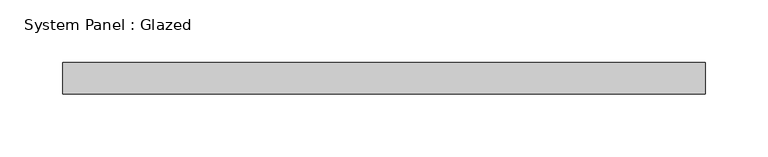
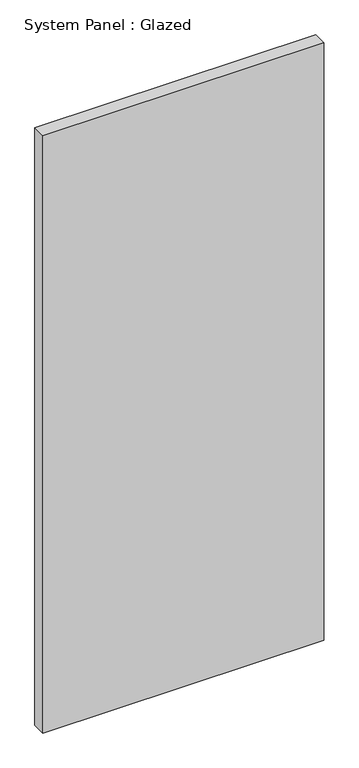
"""IFC4 building model written with IfcOpenShell, lengths in millimetres: plate geometry, System Panel : Glazed."""

from ifc_helpers import new_model, si_unit, origin, origin_with_axes, place, context, project, spatial, polyline, outline, extrude, source, transform, mapped, element, save


def system_panel_glazed_17912afe(model_context):
    return source(origin(), model_context, "Body", "SweptSolid", [
        extrude(outline(polyline([(257.175, 19.05), (-257.175, 19.05), (-257.175, 44.45), (257.175, 44.45), (257.175, 19.05)])), origin_with_axes(), (0.0, 0.0, 1.0), 1155.7),
    ])


if __name__ == "__main__":
    model = new_model("IFC4")
    model_context = context("Model", 3, world=origin())
    ifc_project = project(units=[si_unit("LENGTHUNIT", "METRE", prefix="MILLI")], contexts=[model_context])
    site = spatial("IfcSite", under=ifc_project)
    building = spatial("IfcBuilding", under=site)
    placement = place(None, origin())
    system_panel_glazed_shape = system_panel_glazed_17912afe(model_context)
    element("IfcPlate", 1, ObjectType="System Panel : Glazed", at=placement, inside=building, context=model_context, shape_type="MappedRepresentation", body=[
        mapped(system_panel_glazed_shape, transform((0.0, 0.0, 0.0), x_axis=(1.0, 0.0, 0.0), y_axis=(0.0, 1.0, 0.0), z_axis=(0.0, 0.0, 1.0))),
    ])
    save(model, "model.ifc")

# Revit data of these elements
# Type "System Panel : Glazed"
#   Construction Type Id = "GSP4R"
#   Analytic Construction = "1/8 in Pilkington single glazing"
#   Visual Light Transmittance = 0.9
#   Solar Heat Gain Coefficient = 0.86
#   Heat Transfer Coefficient (U) = 1.18115 BTU/(h·ft²·°F)
#   Define Thermal Properties by = 1
# Element 1 (IfcPlate, "System Panel : Glazed")
#   Materials on its faces: "Glass"
# Materials
#   "Glass": class "Glass", colour RGB 0 128 192, transparency 0.75, Description = "Soda Lime Glass", Cost = 0
